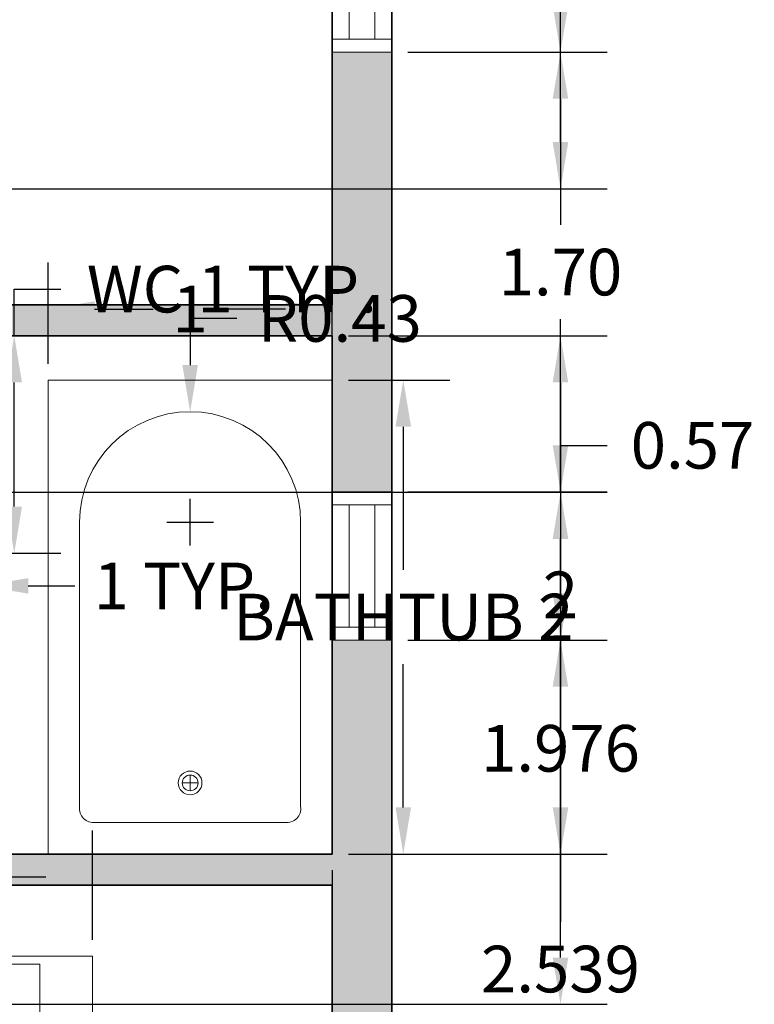
# Model space of a CAD drawing. Units: metres. Extents: x 35.2 to 46.4, y 446.1 to 460.8.
# Tile 4 of 6: x 43.5 to 46.4, y 449.7 to 453.5. Entities that reach past the tile are written whole.
import ezdxf

# ---------------------------------------------------------------- set-up
doc = ezdxf.new("R2010")
doc.units = ezdxf.units.M
for name, color, linetype, lineweight in [('A-ANNO-DIMS', 2, 'Continuous', 18), ('A-GLAZ', 4, 'Continuous', 18), ('A-WALL', 7, 'Continuous', 35), ('A-WALL-PATT', 252, 'Continuous', 13), ('FURNITURE', 53, 'Continuous', 18), ('SANITARY', 151, 'Continuous', 18)]:
    doc.layers.add(name, color=color, linetype=linetype, lineweight=lineweight)
doc.styles.get("Standard").update_dxf_attribs({"font": 'calibri.ttf'})
doc.dimstyles.get("Standard").update_dxf_attribs({"dimtxt": 0.18, "dimasz": 0.18, "dimexe": 0.18, "dimexo": 0.0625, "dimgap": 0.09, "dimtad": 0, "dimtih": 1, "dimtoh": 1, "dimdec": 4, "dimzin": 0, "dimdsep": 46, "dimtxsty": 'Standard', "dimcen": 0.09, "dimadec": 0, "dimazin": 0, "dimtfac": 1, "dimtdec": 4, "dimtofl": 0, "dimtmove": 0, "dimatfit": 3, "dimfxl": 1, "dimtolj": 1, "dimtzin": 0, "dimarcsym": 0})

# ---------------------------------------------------------------- blocks, each defined once
blk = doc.blocks.new('Bath Tub - 26 x 60 in.')
for p, q in [((9, -17), (9, -19)), ((8, -18), (10, -18))]:
    blk.add_line(p, q)
blk.add_lwpolyline([(0, -36), (0, 0), (60, 0), (60, -36)], close=True)
for points in [[(6, -4), (42, -4)], [(4, -30), (4, -6)], [(42, -32), (6, -32)]]:
    blk.add_lwpolyline(points)
for radius in [1.5, 1]:
    blk.add_circle((9, -18), radius)
for centre, radius, start, end in [((5.75, -5.75), 1.77, 81.8699, 188.1301), ((42, -18), 14, 270, 90), ((5.75, -30.25), 1.77, 171.8699, 278.1301)]:
    blk.add_arc(centre, radius, start, end)
blk = doc.blocks.new('Bed - Queen')
for p, q in [((0, -80.00003), (0, 0)), ((0, 0), (59.99999, 0)), ((59.99999, 0), (59.99999, -80.00003)), ((7.99999, -1.2), (28.79998, -1.2)), ((7.99999, -14.4), (7.99999, -1.2)), ((28.79998, -1.2), (28.79998, -14.4)), ((31.19999, -1.2), (51.99999, -1.2)), ((31.19999, -14.4), (31.19999, -1.2)), ((51.99999, -1.2), (51.99999, -16.4)), ((0, -14.4), (44.8, -14.4)), ((59.99999, -29.6), (44.8, -14.4)), ((44.8, -14.4), (44.8, -29.6)), ((51.99999, -16.4), (46.79936, -16.4)), ((44.8, -16.8), (0, -16.8)), ((44.8, -29.6), (59.99999, -29.6)), ((59.99999, -80.00003), (0, -80.00003))]:
    blk.add_line(p, q)
blk = doc.blocks.new('WIN-1172')
for p, q in [((0, 1.1716), (0.23, 1.1716)), ((0, 1.1716), (0, 0)), ((0.23, 1.1716), (0.23, 0)), ((0, 1.1216), (0.23, 1.1216)), ((0.065, 1.1216), (0.065, 0.05)), ((0.165, 1.1216), (0.165, 0.05)), ((0.23, 0.05), (0, 0.05)), ((0.23, 0), (0, 0))]:
    blk.add_line(p, q)
blk = doc.blocks.new('WIN-572')
for p, q in [((0, 0.5716), (0.23, 0.5716)), ((0, 0.5716), (0, 0)), ((0.23, 0.5716), (0.23, 0)), ((0, 0.5216), (0.23, 0.5216)), ((0.065, 0.5216), (0.065, 0.05)), ((0.165, 0.5216), (0.165, 0.05)), ((0.23, 0.05), (0, 0.05)), ((0.23, 0), (0, 0))]:
    blk.add_line(p, q)
blk = doc.blocks.new('*D132')
at = {"layer": 'A-ANNO-DIMS', "color": 0, "lineweight": -2, "transparency": 16777216}
for p, q in [((42.3065, 449.9231), (42.3065, 450.3454)), ((43.8305, 449.9231), (43.8305, 450.3454)), ((42.4865, 450.1654), (42.6457, 450.1654)), ((43.6505, 450.1654), (43.4913, 450.1654))]:
    blk.add_line(p, q, dxfattribs=at)
at = {"layer": 'A-ANNO-DIMS', "color": 0, "transparency": 16777216}
for points in [[(42.4865, 450.1954), (42.4865, 450.1354), (42.3065, 450.1654)], [(43.6505, 450.1954), (43.6505, 450.1354), (43.8305, 450.1654)]]:
    blk.add_solid(points, dxfattribs=at)
at = {"layer": 'Defpoints', "color": 0, "transparency": 16777216}
for p in [(43.8305, 450.1654), (42.3065, 449.8606), (43.8305, 449.8606)]:
    blk.add_point(p, dxfattribs=at)
at = {"layer": 'A-ANNO-DIMS', "color": 0, "transparency": 16777216, "insert": (43.0685, 450.1654), "char_height": 0.18, "attachment_point": 5}
blk.add_mtext('\\A1;2 TYP.', dxfattribs=at)
blk = doc.blocks.new('*D135')
at = {"layer": 'A-ANNO-DIMS', "color": 0, "lineweight": -2, "transparency": 16777216}
for p, q in [((43.5288, 452.2548), (43.5288, 452.4348)), ((43.5288, 452.4348), (43.7088, 452.4348)), ((43.4654, 452.2548), (43.7088, 452.2548)), ((43.5288, 451.5954), (43.5288, 452.0748)), ((43.4654, 451.4154), (43.7088, 451.4154))]:
    blk.add_line(p, q, dxfattribs=at)
at = {"layer": 'A-ANNO-DIMS', "color": 0, "transparency": 16777216}
for points in [[(43.4988, 452.0748), (43.5588, 452.0748), (43.5288, 452.2548)], [(43.4988, 451.5954), (43.5588, 451.5954), (43.5288, 451.4154)]]:
    blk.add_solid(points, dxfattribs=at)
at = {"layer": 'Defpoints', "color": 0, "transparency": 16777216}
for p in [(43.4029, 452.2548), (43.5288, 452.2548), (43.4029, 451.4154)]:
    blk.add_point(p, dxfattribs=at)
at = {"layer": 'A-ANNO-DIMS', "color": 0, "transparency": 16777216, "insert": (44.3691, 452.4348), "char_height": 0.18, "attachment_point": 5}
blk.add_mtext('\\A1;WC 1 TYP.', dxfattribs=at)
blk = doc.blocks.new('*D136')
at = {"layer": 'A-ANNO-DIMS', "color": 0, "lineweight": -2, "transparency": 16777216}
for p, q in [((42.8695, 451.3529), (42.8695, 451.1095)), ((43.4029, 451.3529), (43.4029, 451.1095)), ((42.6895, 451.2895), (42.5095, 451.2895)), ((43.5829, 451.2895), (43.7629, 451.2895))]:
    blk.add_line(p, q, dxfattribs=at)
at = {"layer": 'A-ANNO-DIMS', "color": 0, "transparency": 16777216}
for points in [[(42.6895, 451.3195), (42.6895, 451.2595), (42.8695, 451.2895)], [(43.5829, 451.3195), (43.5829, 451.2595), (43.4029, 451.2895)]]:
    blk.add_solid(points, dxfattribs=at)
at = {"layer": 'Defpoints', "color": 0, "transparency": 16777216}
for p in [(42.8695, 451.4154), (43.4029, 451.4154), (43.4029, 451.2895)]:
    blk.add_point(p, dxfattribs=at)
at = {"layer": 'A-ANNO-DIMS', "color": 0, "transparency": 16777216, "insert": (44.1815, 451.2895), "char_height": 0.18, "attachment_point": 5}
blk.add_mtext('\\A1;1 TYP.', dxfattribs=at)
blk = doc.blocks.new('*D149')
at = {"layer": 'A-ANNO-DIMS', "color": 0, "lineweight": -2, "transparency": 16777216}
for p, q in [((44.8191, 452.0836), (45.2109, 452.0836)), ((45.0309, 451.9036), (45.0309, 451.3514)), ((45.0309, 450.4348), (45.0309, 450.987)), ((44.8191, 450.2548), (45.2109, 450.2548))]:
    blk.add_line(p, q, dxfattribs=at)
at = {"layer": 'A-ANNO-DIMS', "color": 0, "transparency": 16777216}
for points in [[(45.0009, 451.9036), (45.0609, 451.9036), (45.0309, 452.0836)], [(45.0009, 450.4348), (45.0609, 450.4348), (45.0309, 450.2548)]]:
    blk.add_solid(points, dxfattribs=at)
at = {"layer": 'Defpoints', "color": 0, "transparency": 16777216}
for p in [(44.7566, 452.0836), (45.0309, 452.0836), (44.7566, 450.2548)]:
    blk.add_point(p, dxfattribs=at)
at = {"layer": 'A-ANNO-DIMS', "color": 0, "transparency": 16777216, "insert": (45.0309, 451.1692), "char_height": 0.18, "attachment_point": 5}
blk.add_mtext('\\A1;BATHTUB 2', dxfattribs=at)
blk = doc.blocks.new('*D150')
at = {"layer": 'A-ANNO-DIMS', "color": 0, "lineweight": -2, "transparency": 16777216}
for p, q in [((43.6593, 452.1461), (43.6593, 452.5379)), ((44.7566, 452.1461), (44.7566, 452.5379)), ((43.8393, 452.3579), (44.0658, 452.3579)), ((44.5766, 452.3579), (44.3501, 452.3579))]:
    blk.add_line(p, q, dxfattribs=at)
at = {"layer": 'A-ANNO-DIMS', "color": 0, "transparency": 16777216}
for points in [[(43.8393, 452.3879), (43.8393, 452.3279), (43.6593, 452.3579)], [(44.5766, 452.3879), (44.5766, 452.3279), (44.7566, 452.3579)]]:
    blk.add_solid(points, dxfattribs=at)
at = {"layer": 'Defpoints', "color": 0, "transparency": 16777216}
for p in [(43.6593, 452.3579), (43.6593, 452.0836), (44.7566, 452.0836)]:
    blk.add_point(p, dxfattribs=at)
at = {"layer": 'A-ANNO-DIMS', "color": 0, "transparency": 16777216, "insert": (44.208, 452.3579), "char_height": 0.18, "attachment_point": 5}
blk.add_mtext('\\A1;1', dxfattribs=at)
blk = doc.blocks.new('*D155')
at = {"layer": 'A-ANNO-DIMS', "color": 0, "lineweight": -2, "transparency": 16777216}
for p, q in [((37.8991, 451.6506), (45.8178, 451.6506)), ((45.6378, 451.4706), (45.6378, 450.8449)), ((45.6378, 449.8548), (45.6378, 450.4805)), ((37.8991, 449.6748), (45.8178, 449.6748))]:
    blk.add_line(p, q, dxfattribs=at)
at = {"layer": 'A-ANNO-DIMS', "color": 0, "transparency": 16777216}
for points in [[(45.6078, 451.4706), (45.6678, 451.4706), (45.6378, 451.6506)], [(45.6078, 449.8548), (45.6678, 449.8548), (45.6378, 449.6748)]]:
    blk.add_solid(points, dxfattribs=at)
at = {"layer": 'Defpoints', "color": 0, "transparency": 16777216}
for p in [(37.8366, 451.6506), (45.6378, 451.6506), (37.8366, 449.6748)]:
    blk.add_point(p, dxfattribs=at)
at = {"layer": 'A-ANNO-DIMS', "color": 0, "transparency": 16777216, "insert": (45.6378, 450.6627), "char_height": 0.18, "attachment_point": 5}
blk.add_mtext('\\A1;1.976', dxfattribs=at)
blk = doc.blocks.new('*D156')
at = {"layer": 'A-ANNO-DIMS', "color": 0, "lineweight": -2, "transparency": 16777216}
for p, q in [((37.8991, 455.122), (45.8178, 455.122)), ((45.6378, 454.942), (45.6378, 454.1543)), ((45.6378, 453.0022), (45.6378, 453.7898)), ((37.8991, 452.8222), (45.8178, 452.8222))]:
    blk.add_line(p, q, dxfattribs=at)
at = {"layer": 'A-ANNO-DIMS', "color": 0, "transparency": 16777216}
for points in [[(45.6078, 454.942), (45.6678, 454.942), (45.6378, 455.122)], [(45.6078, 453.0022), (45.6678, 453.0022), (45.6378, 452.8222)]]:
    blk.add_solid(points, dxfattribs=at)
at = {"layer": 'Defpoints', "color": 0, "transparency": 16777216}
for p in [(37.8366, 455.122), (45.6378, 455.122), (37.8366, 452.8222)]:
    blk.add_point(p, dxfattribs=at)
at = {"layer": 'A-ANNO-DIMS', "color": 0, "transparency": 16777216, "insert": (45.6378, 453.9721), "char_height": 0.18, "attachment_point": 5}
blk.add_mtext('\\A1;2.3', dxfattribs=at)
blk = doc.blocks.new('*D161')
at = {"layer": 'A-ANNO-DIMS', "color": 0, "lineweight": -2, "transparency": 16777216}
for p, q in [((45.0491, 451.0803), (45.8178, 451.0803)), ((45.6378, 450.9003), (45.6378, 449.9931)), ((45.6378, 448.7214), (45.6378, 449.6286)), ((45.0491, 448.5414), (45.8178, 448.5414))]:
    blk.add_line(p, q, dxfattribs=at)
at = {"layer": 'A-ANNO-DIMS', "color": 0, "transparency": 16777216}
for points in [[(45.6078, 450.9003), (45.6678, 450.9003), (45.6378, 451.0803)], [(45.6078, 448.7214), (45.6678, 448.7214), (45.6378, 448.5414)]]:
    blk.add_solid(points, dxfattribs=at)
at = {"layer": 'Defpoints', "color": 0, "transparency": 16777216}
for p in [(44.9866, 451.0803), (45.6378, 451.0803), (44.9866, 448.5414)]:
    blk.add_point(p, dxfattribs=at)
at = {"layer": 'A-ANNO-DIMS', "color": 0, "transparency": 16777216, "insert": (45.6378, 449.8109), "char_height": 0.18, "attachment_point": 5}
blk.add_mtext('\\A1;2.539', dxfattribs=at)
blk = doc.blocks.new('*D162')
at = {"layer": 'A-ANNO-DIMS', "color": 0, "lineweight": -2, "transparency": 16777216}
for p, q in [((45.6378, 451.6519), (45.6378, 451.8319)), ((45.6378, 451.8319), (45.8178, 451.8319)), ((45.0491, 451.6519), (45.8178, 451.6519)), ((45.6378, 451.2603), (45.6378, 451.4719)), ((45.0491, 451.0803), (45.8178, 451.0803))]:
    blk.add_line(p, q, dxfattribs=at)
at = {"layer": 'A-ANNO-DIMS', "color": 0, "transparency": 16777216}
for points in [[(45.6078, 451.4719), (45.6678, 451.4719), (45.6378, 451.6519)], [(45.6078, 451.2603), (45.6678, 451.2603), (45.6378, 451.0803)]]:
    blk.add_solid(points, dxfattribs=at)
at = {"layer": 'Defpoints', "color": 0, "transparency": 16777216}
for p in [(44.9866, 451.6519), (45.6378, 451.6519), (44.9866, 451.0803)]:
    blk.add_point(p, dxfattribs=at)
at = {"layer": 'A-ANNO-DIMS', "color": 0, "transparency": 16777216, "insert": (46.1476, 451.8319), "char_height": 0.18, "attachment_point": 5}
blk.add_mtext('\\A1;0.57', dxfattribs=at)
blk = doc.blocks.new('*D163')
at = {"layer": 'A-ANNO-DIMS', "color": 0, "lineweight": -2, "transparency": 16777216}
for p, q in [((45.0491, 453.3493), (45.8178, 453.3493)), ((45.6378, 453.1693), (45.6378, 452.6828)), ((45.6378, 451.8319), (45.6378, 452.3184)), ((45.0491, 451.6519), (45.8178, 451.6519))]:
    blk.add_line(p, q, dxfattribs=at)
at = {"layer": 'A-ANNO-DIMS', "color": 0, "transparency": 16777216}
for points in [[(45.6078, 453.1693), (45.6678, 453.1693), (45.6378, 453.3493)], [(45.6078, 451.8319), (45.6678, 451.8319), (45.6378, 451.6519)]]:
    blk.add_solid(points, dxfattribs=at)
at = {"layer": 'Defpoints', "color": 0, "transparency": 16777216}
for p in [(44.9866, 453.3493), (45.6378, 453.3493), (44.9866, 451.6519)]:
    blk.add_point(p, dxfattribs=at)
at = {"layer": 'A-ANNO-DIMS', "color": 0, "transparency": 16777216, "insert": (45.6378, 452.5006), "char_height": 0.18, "attachment_point": 5}
blk.add_mtext('\\A1;1.70', dxfattribs=at)
blk = doc.blocks.new('*D164')
at = {"layer": 'A-ANNO-DIMS', "color": 0, "lineweight": -2, "transparency": 16777216}
for p, q in [((45.0491, 454.5208), (45.8178, 454.5208)), ((45.6378, 454.3408), (45.6378, 454.1159)), ((45.6378, 453.5293), (45.6378, 453.7542)), ((45.0491, 453.3493), (45.8178, 453.3493))]:
    blk.add_line(p, q, dxfattribs=at)
at = {"layer": 'A-ANNO-DIMS', "color": 0, "transparency": 16777216}
for points in [[(45.6078, 454.3408), (45.6678, 454.3408), (45.6378, 454.5208)], [(45.6078, 453.5293), (45.6678, 453.5293), (45.6378, 453.3493)]]:
    blk.add_solid(points, dxfattribs=at)
at = {"layer": 'Defpoints', "color": 0, "transparency": 16777216}
for p in [(44.9866, 454.5208), (45.6378, 454.5208), (44.9866, 453.3493)]:
    blk.add_point(p, dxfattribs=at)
at = {"layer": 'A-ANNO-DIMS', "color": 0, "transparency": 16777216, "insert": (45.6378, 453.9351), "char_height": 0.18, "attachment_point": 5}
blk.add_mtext('\\A1;1.17', dxfattribs=at)
blk = doc.blocks.new('*D171')
at = {"layer": 'A-ANNO-DIMS', "color": 0, "lineweight": -2, "transparency": 16777216}
for p, q in [((42.1191, 450.1923), (42.1191, 446.0736)), ((44.7566, 450.1923), (44.7566, 446.0736)), ((42.2991, 446.2536), (43.1085, 446.2536)), ((44.5766, 446.2536), (43.7673, 446.2536))]:
    blk.add_line(p, q, dxfattribs=at)
at = {"layer": 'A-ANNO-DIMS', "color": 0, "transparency": 16777216}
for points in [[(42.2991, 446.2836), (42.2991, 446.2236), (42.1191, 446.2536)], [(44.5766, 446.2836), (44.5766, 446.2236), (44.7566, 446.2536)]]:
    blk.add_solid(points, dxfattribs=at)
at = {"layer": 'Defpoints', "color": 0, "transparency": 16777216}
for p in [(42.1191, 450.2548), (44.7566, 450.2548), (44.7566, 446.2536)]:
    blk.add_point(p, dxfattribs=at)
at = {"layer": 'A-ANNO-DIMS', "color": 0, "transparency": 16777216, "insert": (43.4379, 446.2536), "char_height": 0.18, "attachment_point": 5}
blk.add_mtext('\\A1;2.64', dxfattribs=at)
blk = doc.blocks.new('*D172')
at = {"layer": 'A-ANNO-DIMS', "color": 0, "lineweight": -2, "transparency": 16777216}
for p, q in [((44.819095, 452.254779), (45.817795, 452.254779)), ((45.637795, 452.074779), (45.637795, 451.435679)), ((45.637795, 450.434779), (45.637795, 451.073879)), ((44.819095, 450.254779), (45.817795, 450.254779))]:
    blk.add_line(p, q, dxfattribs=at)
at = {"layer": 'A-ANNO-DIMS', "color": 0, "transparency": 16777216}
for points in [[(45.607795, 452.074779), (45.667795, 452.074779), (45.637795, 452.254779)], [(45.607795, 450.434779), (45.667795, 450.434779), (45.637795, 450.254779)]]:
    blk.add_solid(points, dxfattribs=at)
at = {"layer": 'Defpoints', "color": 0, "transparency": 16777216}
for p in [(44.756595, 452.254779), (45.637795, 452.254779), (44.756595, 450.254779)]:
    blk.add_point(p, dxfattribs=at)
at = {"layer": 'A-ANNO-DIMS', "color": 0, "transparency": 16777216, "insert": (45.637795, 451.254779), "char_height": 0.18, "attachment_point": 5}
blk.add_mtext('\\A1;2', dxfattribs=at)
blk = doc.blocks.new('*D175')
at = {"layer": 'A-ANNO-DIMS', "color": 0, "lineweight": -2, "transparency": 16777216}
for p, q in [((44.7566, 451.1428), (44.7566, 460.756)), ((44.9866, 451.1428), (44.9866, 460.756)), ((44.5766, 460.576), (44.3966, 460.576)), ((45.1666, 460.576), (45.3466, 460.576))]:
    blk.add_line(p, q, dxfattribs=at)
at = {"layer": 'A-ANNO-DIMS', "color": 0, "transparency": 16777216}
for points in [[(44.5766, 460.606), (44.5766, 460.546), (44.7566, 460.576)], [(45.1666, 460.606), (45.1666, 460.546), (44.9866, 460.576)]]:
    blk.add_solid(points, dxfattribs=at)
at = {"layer": 'Defpoints', "color": 0, "transparency": 16777216}
for p in [(44.9866, 460.576), (44.7566, 451.0803), (44.9866, 451.0803)]:
    blk.add_point(p, dxfattribs=at)
at = {"layer": 'A-ANNO-DIMS', "color": 0, "transparency": 16777216, "insert": (45.6744, 460.576), "char_height": 0.18, "attachment_point": 5}
blk.add_mtext('\\A1;0.23', dxfattribs=at)
blk = doc.blocks.new('*D189')
at = {"layer": 'A-ANNO-DIMS', "color": 0, "lineweight": -2, "transparency": 16777216}
for p, q in [((44.388, 452.3217), (44.208, 452.3217)), ((44.208, 452.3217), (44.208, 452.1417)), ((44.208, 451.4449), (44.208, 451.6249)), ((44.118, 451.5349), (44.298, 451.5349))]:
    blk.add_line(p, q, dxfattribs=at)
at = {"layer": 'A-ANNO-DIMS', "color": 0, "transparency": 16777216}
blk.add_solid([(44.178, 452.1417), (44.238, 452.1417), (44.208, 451.9617)], dxfattribs=at)
at = {"layer": 'Defpoints', "color": 0, "transparency": 16777216}
for p in [(44.208, 451.9617), (44.208, 451.5349)]:
    blk.add_point(p, dxfattribs=at)
at = {"layer": 'A-ANNO-DIMS', "color": 0, "transparency": 16777216, "insert": (44.7859, 452.3217), "char_height": 0.18, "attachment_point": 5}
blk.add_mtext('\\A1;R0.43', dxfattribs=at)

msp = doc.modelspace()

# ---------------------------------------------------------------- hatches: boundary and pattern name
at = {"layer": 'A-WALL-PATT'}
h = msp.add_hatch(color=256, dxfattribs=at)
h.dxf.hatch_style = 1
h.paths.add_polyline_path([(44.9866, 457.1611), (44.7566, 457.1611), (44.7566, 454.5208), (44.9866, 454.5208)])
h.paths.add_polyline_path([(44.9866, 453.3493), (44.7566, 453.3493), (44.7566, 452.3748), (42.8766, 452.3748), (42.8766, 452.8748), (42.1191, 452.8748), (42.1191, 452.9307), (41.9991, 452.9307), (41.9991, 452.2548), (42.1191, 452.2548), (42.1191, 452.7548), (42.7566, 452.7548), (42.7566, 452.2548), (44.7566, 452.2548), (44.7566, 451.6519), (44.9866, 451.6519)])
h.paths.add_polyline_path([(44.9866, 451.0803), (44.7566, 451.0803), (44.7566, 450.2548), (43.6593, 450.2548), (43.0598, 450.2548, -0.016107), (43.0354, 450.2548), (42.1191, 450.2548), (42.1191, 450.7446), (41.9991, 450.7446), (41.9991, 450.2548), (41.8662, 450.2548), (41.8662, 450.1348), (44.7566, 450.1348), (44.7566, 448.5414), (44.9866, 448.5414)])
h.paths.add_polyline_path([(44.9866, 447.3698), (44.7566, 447.3698), (44.7566, 447.1348), (41.1566, 447.1348), (41.1566, 450.1348), (41.2566, 450.1348), (41.2566, 450.2548), (41.0366, 450.2548), (41.0366, 446.9048), (44.9866, 446.9048)])

# ---------------------------------------------------------------- linework, layer by layer
at = {"layer": 'A-WALL'}
for p, q in [((44.9866, 459.9248), (44.9866, 446.9048)), ((44.7566, 459.6948), (44.7566, 452.3748)), ((42.8766, 452.3748), (44.7566, 452.3748)), ((41.9991, 452.2548), (44.7566, 452.2548)), ((44.7566, 452.2548), (44.7566, 450.2548)), ((42.1191, 450.2548), (44.7566, 450.2548)), ((41.8662, 450.1348), (44.7566, 450.1348)), ((44.7566, 450.1348), (44.7566, 447.1348))]:
    msp.add_line(p, q, dxfattribs=at)

# ---------------------------------------------------------------- block references
at = {"layer": 'A-GLAZ'}
for name, p in [('WIN-1172', (44.7566, 453.3493)), ('WIN-572', (44.7566, 451.0803))]:
    msp.add_blockref(name, p, dxfattribs=at)
at = {"layer": 'FURNITURE', "transparency": 33554521, "xscale": 0.0254, "yscale": 0.0254, "zscale": 0.0254}
msp.add_blockref('Bed - Queen', (42.3065, 449.8606), dxfattribs=at)
at = {"layer": 'SANITARY', "transparency": 33554521, "xscale": 0.03048, "yscale": 0.03048, "zscale": 0.03048, "rotation": 90}
msp.add_blockref('Bath Tub - 26 x 60 in.', (43.6593, 450.2548), dxfattribs=at)

# ---------------------------------------------------------------- dimensions: what is measured, and where the dimension line sits
at = {"layer": 'A-ANNO-DIMS'}
for base, p1, p2, picture, middle in [((44.9866, 460.576), (44.7566, 451.0803), (44.9866, 451.0803), '*D175', (45.6744, 460.576)), ((44.7566, 446.2536), (42.1191, 450.2548), (44.7566, 450.2548), '*D171', (43.4379, 446.2536))]:
    dim = msp.add_linear_dim(base=base, p1=p1, p2=p2, dimstyle='Standard', override={"dimdec": 2, "dimlfac": 1, "dimrnd": 0, "dimzin": 0, "dimdsep": 46, "dimlunit": 2}, dxfattribs=at)
    dim.commit()
    dim.dimension.update_dxf_attribs({"geometry": picture, "text_midpoint": middle})
for base, p1, p2, angle, override, picture, middle in [((45.6378, 455.122), (37.8366, 452.8222), (37.8366, 455.122), 90, {"dimdec": 1, "dimlfac": 1, "dimrnd": 0, "dimzin": 0, "dimdsep": 46, "dimlunit": 2}, '*D156', (45.6378, 453.9721)), ((45.6378, 454.5208), (44.9866, 453.3493), (44.9866, 454.5208), 90, {"dimdec": 2, "dimlfac": 1, "dimrnd": 0, "dimzin": 0, "dimdsep": 46, "dimlunit": 2}, '*D164', (45.6378, 453.9351)), ((45.6378, 453.3493), (44.9866, 451.6519), (44.9866, 453.3493), 90, {"dimdec": 2, "dimlfac": 1, "dimrnd": 0, "dimzin": 0, "dimdsep": 46, "dimlunit": 2}, '*D163', (45.6378, 452.5006)), ((43.6593, 452.3579), (44.7566, 452.0836), (43.6593, 452.0836), 180, {"dimdec": 0, "dimlfac": 1, "dimrnd": 0, "dimzin": 0, "dimdsep": 46, "dimlunit": 2}, '*D150', (44.208, 452.3579)), ((45.6378, 452.2548), (44.7566, 450.2548), (44.7566, 452.2548), 90, {"dimdec": 0, "dimlfac": 1, "dimrnd": 0, "dimzin": 0, "dimdsep": 46, "dimlunit": 2}, '*D172', (45.6378, 451.2548)), ((45.6378, 451.6519), (44.9866, 451.0803), (44.9866, 451.6519), 90, {"dimdec": 2, "dimlfac": 1, "dimrnd": 0, "dimzin": 0, "dimdsep": 46, "dimlunit": 2}, '*D162', (46.1476, 451.8319)), ((45.6378, 451.6506), (37.8366, 449.6748), (37.8366, 451.6506), 90, {"dimdec": 3, "dimlfac": 1, "dimrnd": 0, "dimzin": 0, "dimdsep": 46, "dimlunit": 2}, '*D155', (45.6378, 450.6627)), ((45.6378, 451.0803), (44.9866, 448.5414), (44.9866, 451.0803), 90, {"dimdec": 3, "dimlfac": 1, "dimrnd": 0, "dimzin": 0, "dimdsep": 46, "dimlunit": 2}, '*D161', (45.6378, 449.8109))]:
    dim = msp.add_linear_dim(base=base, p1=p1, p2=p2, angle=angle, dimstyle='Standard', override=override, dxfattribs=at)
    dim.commit()
    dim.dimension.update_dxf_attribs({"geometry": picture, "text_midpoint": middle})
for base, p1, p2, text, picture, middle in [((43.5288, 452.2548), (43.4029, 451.4154), (43.4029, 452.2548), 'WC <> TYP.', '*D135', (44.3691, 452.4348)), ((45.0309, 452.0836), (44.7566, 450.2548), (44.7566, 452.0836), 'BATHTUB <>', '*D149', (45.0309, 451.1692))]:
    dim = msp.add_linear_dim(base=base, p1=p1, p2=p2, angle=90, text=text, dimstyle='Standard', override={"dimdec": 0, "dimlfac": 1, "dimrnd": 0, "dimzin": 0, "dimdsep": 46, "dimlunit": 2}, dxfattribs=at)
    dim.commit()
    dim.dimension.update_dxf_attribs({"geometry": picture, "text_midpoint": middle})
dim = msp.add_radius_dim(center=(44.208, 451.5349), mpoint=(44.208, 451.9617), dimstyle='Standard', override={"dimdec": 2, "dimlfac": 1, "dimrnd": 0, "dimzin": 0, "dimdsep": 46, "dimlunit": 2}, dxfattribs=at)
dim.commit()
dim.dimension.update_dxf_attribs({"geometry": '*D189', "text_midpoint": (44.7859, 452.3217)})
for base, p1, p2, picture, middle in [((43.4029, 451.2895), (42.8695, 451.4154), (43.4029, 451.4154), '*D136', (44.1815, 451.2895)), ((43.8305, 450.1654), (42.3065, 449.8606), (43.8305, 449.8606), '*D132', (43.0685, 450.1654))]:
    dim = msp.add_linear_dim(base=base, p1=p1, p2=p2, text='<> TYP.', dimstyle='Standard', override={"dimdec": 0, "dimlfac": 1, "dimrnd": 0, "dimzin": 0, "dimdsep": 46, "dimlunit": 2}, dxfattribs=at)
    dim.commit()
    dim.dimension.update_dxf_attribs({"geometry": picture, "text_midpoint": middle})

doc.saveas('drawing.dxf')
